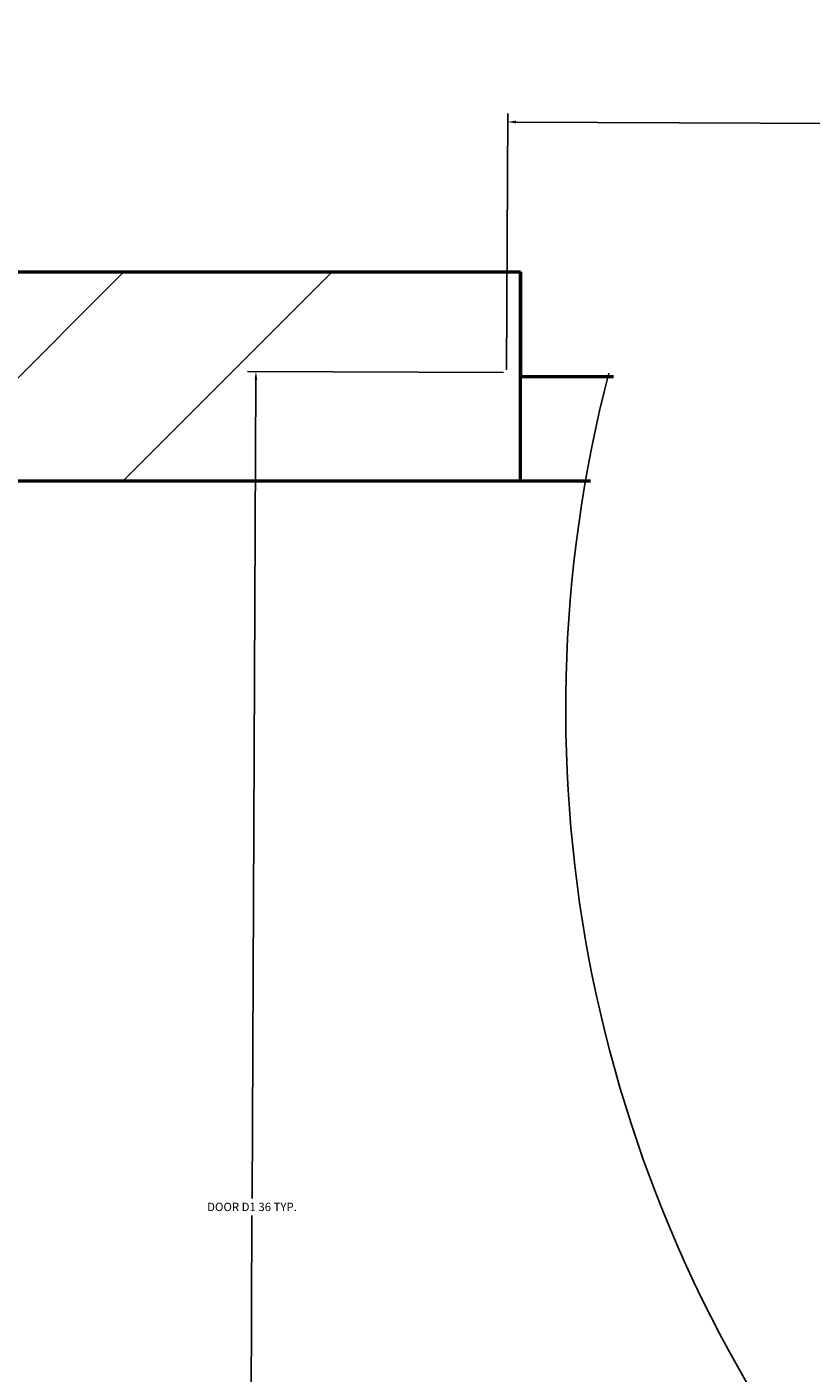
# Model space of a CAD drawing. Units: inches. Extents: x 1901 to 2863, y 888 to 2433.
# Tile 28 of 91: x 2557 to 2573, y 1376 to 1405. Entities that reach past the tile are written whole.
import ezdxf

# ---------------------------------------------------------------- set-up
doc = ezdxf.new("R2010")
doc.units = ezdxf.units.IN
for name, color, linetype, lineweight in [('A-ANNO-DIMS', 2, 'Continuous', 18), ('A-DOOR', 4, 'Continuous', 25), ('A-WALL', 7, 'Continuous', 50), ('A-WALL-PATT', 8, 'Continuous', 13)]:
    doc.layers.add(name, color=color, linetype=linetype, lineweight=lineweight)
doc.styles.get("Standard").update_dxf_attribs({"font": 'arial.ttf'})
doc.dimstyles.get("Standard").update_dxf_attribs({"dimtxt": 0.18, "dimasz": 0.18, "dimexe": 0.18, "dimexo": 0.0625, "dimgap": 0.09, "dimtad": 0, "dimtih": 1, "dimtoh": 1, "dimdec": 4, "dimzin": 0, "dimdsep": 46, "dimtxsty": 'Standard', "dimcen": 0.09, "dimadec": 0, "dimazin": 0, "dimtfac": 1, "dimtdec": 4, "dimtofl": 0, "dimtmove": 0, "dimatfit": 3, "dimfxl": 1, "dimtolj": 1, "dimtzin": 0, "dimarcsym": 0})

# ---------------------------------------------------------------- blocks, each defined once
blk = doc.blocks.new('DOOR-29')
blk.add_arc((-0.004, 7.119), 28.865, 345.6888, 90)
blk = doc.blocks.new('*D31')
at = {"layer": 'A-ANNO-DIMS', "color": 0, "lineweight": -2, "transparency": 16777216}
for p, q in [((2566.77, 1397.965), (2561.253, 1397.99)), ((2561.432, 1397.81), (2561.35, 1380.173)), ((2561.266, 1362.17), (2561.348, 1379.807)), ((2566.603, 1361.965), (2561.085, 1361.991))]:
    blk.add_line(p, q, dxfattribs=at)
at = {"layer": 'A-ANNO-DIMS', "color": 0, "transparency": 16777216}
for points in [[(2561.402, 1397.81), (2561.462, 1397.809), (2561.433, 1397.99)], [(2561.236, 1362.17), (2561.296, 1362.17), (2561.265, 1361.99)]]:
    blk.add_solid(points, dxfattribs=at)
at = {"layer": 'Defpoints', "color": 0, "transparency": 16777216}
for p in [(2566.833, 1397.964), (2561.265, 1361.99), (2566.665, 1361.965)]:
    blk.add_point(p, dxfattribs=at)
at = {"layer": 'A-ANNO-DIMS', "color": 0, "transparency": 16777216, "insert": (2561.349, 1379.99), "char_height": 0.18, "attachment_point": 5}
blk.add_mtext('\\A1;DOOR D1 36 TYP.', dxfattribs=at)
blk = doc.blocks.new('*D32')
at = {"layer": 'A-ANNO-DIMS', "color": 0, "lineweight": -2, "transparency": 16777216}
for p, q in [((2566.833, 1398.027), (2566.858, 1403.544)), ((2567.038, 1403.364), (2581.416, 1403.297)), ((2596.85, 1403.225), (2582.472, 1403.292)), ((2597.005, 1397.887), (2597.03, 1403.404))]:
    blk.add_line(p, q, dxfattribs=at)
at = {"layer": 'A-ANNO-DIMS', "color": 0, "transparency": 16777216}
for points in [[(2567.038, 1403.394), (2567.037, 1403.334), (2566.858, 1403.364)], [(2596.85, 1403.255), (2596.849, 1403.195), (2597.03, 1403.224)]]:
    blk.add_solid(points, dxfattribs=at)
at = {"layer": 'Defpoints', "color": 0, "transparency": 16777216}
for p in [(2566.858, 1403.364), (2566.833, 1397.964), (2597.005, 1397.824)]:
    blk.add_point(p, dxfattribs=at)
at = {"layer": 'A-ANNO-DIMS', "color": 0, "transparency": 16777216, "insert": (2581.944, 1403.294), "char_height": 0.18, "attachment_point": 5}
blk.add_mtext('\\A1;30 TYP.', dxfattribs=at)

msp = doc.modelspace()

# ---------------------------------------------------------------- hatches: boundary and pattern name
at = {"layer": 'A-WALL-PATT'}
h = msp.add_hatch(dxfattribs=at)
h.set_pattern_fill('ANSI32', color=256)
h.paths.add_polyline_path([(2443.926, 2139.888), (2439.426, 2139.888), (2439.426, 2069.348), (2441.676, 2069.348), (2443.926, 2069.348), (2443.926, 2078.634), (2521.926, 2078.634), (2521.926, 2075.067), (2524.176, 2075.067), (2526.426, 2075.067), (2526.426, 2078.634), (2571.755, 2078.634), (2571.755, 2080.884), (2571.755, 2083.134), (2443.926, 2083.134)])
h.paths.add_polyline_path([(2526.426, 2054.634), (2524.176, 2054.634), (2521.926, 2054.634), (2521.926, 2030.634), (2443.926, 2030.634), (2443.926, 2045.348), (2439.426, 2045.348), (2439.426, 1983.867), (2443.926, 1983.867), (2443.926, 2026.134), (2521.926, 2026.134), (2526.426, 2026.134)])
h.paths.add_polyline_path([(2443.926, 1923.867), (2439.426, 1923.867), (2439.426, 1872.634), (2443.926, 1872.634)])
h.paths.add_polyline_path([(2636.233, 1766.134), (2609.926, 1766.134), (2609.926, 1779.785), (2605.426, 1779.785), (2605.426, 1766.134), (2486.614, 1766.134), (2486.614, 1770.671), (2482.114, 1770.671), (2482.114, 1766.134), (2482.114, 1761.634), (2636.233, 1761.634), (2636.233, 1763.884)])
h.paths.add_polyline_path([(2519.536, 1663.384), (2519.536, 1665.634), (2494.926, 1665.634), (2481.831, 1665.634), (2481.831, 1663.384), (2481.831, 1661.134), (2490.426, 1661.134), (2490.426, 1640.157), (2494.926, 1640.157), (2494.926, 1661.134), (2519.536, 1661.134)])
h.paths.add_polyline_path([(2443.926, 1712.134), (2443.926, 1716.634), (2414.464, 1716.634), (2414.464, 1712.134), (2439.426, 1712.134), (2439.426, 1545.507), (2443.926, 1545.507), (2443.926, 1661.134), (2448.475, 1661.134), (2448.475, 1665.634), (2443.926, 1665.634)])
h.paths.add_polyline_path([(2343.426, 1712.134), (2365.525, 1712.134), (2365.525, 1714.384), (2365.525, 1716.634), (2333.871, 1716.634), (2333.871, 1714.384), (2333.871, 1712.134), (2338.926, 1712.134), (2338.926, 1575.634), (2338.926, 1545.507), (2343.426, 1545.507), (2343.426, 1547.507), (2343.426, 1580.134)])
h.paths.add_polyline_path([(2752.926, 1665.634), (2579.536, 1665.634), (2579.536, 1661.134), (2615.926, 1661.134), (2615.926, 1529.134), (2598.931, 1529.134), (2598.931, 1524.634), (2623.127, 1524.634), (2623.127, 1526.884), (2623.127, 1529.134), (2620.426, 1529.134), (2620.426, 1661.134), (2748.426, 1661.134), (2748.426, 1633.499), (2752.926, 1633.499)])
h.paths.add_polyline_path([(2752.926, 1419.929), (2748.426, 1419.929), (2748.426, 1400.134), (2659.426, 1400.134), (2659.426, 1444.333), (2657.176, 1444.333), (2654.926, 1444.333), (2654.926, 1400.134), (2643.649, 1400.134), (2643.649, 1395.634), (2748.426, 1395.634), (2748.426, 1364.035), (2752.926, 1364.035)])
h.paths.add_polyline_path([(2752.926, 1492.878), (2748.426, 1492.878), (2748.426, 1476.634), (2667.426, 1476.634), (2667.426, 1479.71), (2665.176, 1479.71), (2662.926, 1479.71), (2662.926, 1476.634), (2654.926, 1476.634), (2654.926, 1469.536), (2659.426, 1469.536), (2659.426, 1472.134), (2748.426, 1472.134), (2748.426, 1455.929), (2752.926, 1455.929)])
h.paths.add_polyline_path([(2752.926, 1304.035), (2748.426, 1304.035), (2748.426, 1263.634), (2738.66, 1263.634), (2738.66, 1259.134), (2752.926, 1259.134)])
h.paths.add_polyline_path([(2685.926, 1259.134), (2695.49, 1259.134), (2695.49, 1261.384), (2695.49, 1263.634), (2677.837, 1263.634), (2677.837, 1261.384), (2677.837, 1259.134), (2681.426, 1259.134), (2681.426, 1203.634), (2653.277, 1203.634), (2653.277, 1199.134), (2685.926, 1199.134), (2685.926, 1203.634)])
h.paths.add_polyline_path([(2609.426, 1395.634), (2611.848, 1395.634), (2611.848, 1400.134), (2598.888, 1400.134), (2598.888, 1397.884), (2598.888, 1395.634), (2604.926, 1395.634), (2604.926, 1268.134), (2554.726, 1268.134), (2554.726, 1265.884), (2554.726, 1263.634), (2604.926, 1263.634), (2604.926, 1203.634), (2571.306, 1203.634), (2571.306, 1199.134), (2604.926, 1199.134), (2629.277, 1199.134), (2629.277, 1201.384), (2629.277, 1203.634), (2609.426, 1203.634), (2609.426, 1258.634), (2609.426, 1259.134), (2654.804, 1259.134), (2654.804, 1263.634), (2609.426, 1263.634)])
h.paths.add_polyline_path([(2443.926, 1304.035), (2439.426, 1304.035), (2439.426, 1259.134), (2443.926, 1259.134), (2456.16, 1259.134), (2456.16, 1261.384), (2456.16, 1263.634), (2443.926, 1263.634)])
h.paths.add_polyline_path([(2525.426, 1263.634), (2531.778, 1263.634), (2531.778, 1268.134), (2520.926, 1268.134), (2520.926, 1263.634), (2511.409, 1263.634), (2511.409, 1259.134), (2520.926, 1259.134), (2520.926, 1199.134), (2547.306, 1199.134), (2547.306, 1201.384), (2547.306, 1203.634), (2525.426, 1203.634)])
h.paths.add_polyline_path([(2443.926, 1434.842), (2439.426, 1434.842), (2439.426, 1364.035), (2441.676, 1364.035), (2443.926, 1364.035)])
h.paths.add_polyline_path([(2567.134, 1400.134), (2443.926, 1400.134), (2443.926, 1395.634), (2567.134, 1395.634)])
h.paths.add_polyline_path([(2443.926, 1545.507), (2439.426, 1545.507), (2439.426, 1494.842), (2443.926, 1494.842)])
h.paths.add_polyline_path([(2494.926, 1553.349), (2492.676, 1553.349), (2490.426, 1553.349), (2490.426, 1524.634), (2494.926, 1524.634), (2525.936, 1524.634), (2525.936, 1526.884), (2525.936, 1529.134), (2494.926, 1529.134)])
h.paths.add_polyline_path([(2752.926, 1573.499), (2748.426, 1573.499), (2748.426, 1529.134), (2657.759, 1529.134), (2657.759, 1524.634), (2662.926, 1524.634), (2662.926, 1498.631), (2667.426, 1498.631), (2667.426, 1524.634), (2748.426, 1524.634), (2748.426, 1516.878), (2752.926, 1516.878)])
h.paths.add_polyline_path([(2038.602, 2237.418), (2080.174, 2237.418), (2080.174, 2256.075), (2038.602, 2256.075)], flags=9)
h.paths.add_polyline_path([(2292.009, 1062.394), (2539.932, 1062.394), (2539.932, 1099.487), (2292.009, 1099.487)], flags=9)
h.paths.add_polyline_path([(2424.91, 1832.253), (2448.513, 1832.253), (2448.513, 1846.678), (2424.91, 1846.678)], flags=9)
h.paths.add_polyline_path([(2359.076, 1832.253), (2382.678, 1832.253), (2382.678, 1846.678), (2359.076, 1846.678)], flags=9)
h.paths.add_polyline_path([(2352.899, 1684.802), (2367.543, 1684.802), (2367.543, 1697.167), (2352.899, 1697.167)], flags=9)
h.paths.add_polyline_path([(2079.288, 1755.826), (2169.024, 1755.826), (2169.024, 1774.372), (2079.288, 1774.372)], flags=9)
h.paths.add_polyline_path([(2404.09, 1373.857), (2404.09, 1463.593), (2385.544, 1463.593), (2385.544, 1373.857)], flags=9)
h.paths.add_polyline_path([(2268.091, 2236.371), (2309.636, 2236.371), (2309.636, 2255.028), (2268.091, 2255.028)], flags=9)
h.paths.add_polyline_path([(2575.96, 1700.951), (2665.696, 1700.951), (2665.696, 1719.498), (2575.96, 1719.498)], flags=9)
h.paths.add_polyline_path([(2302.962, 1878.474), (2329.524, 1878.474), (2329.524, 1888.777), (2302.962, 1888.777)], flags=9)
h.paths.add_polyline_path([(2097.415, 2240.576), (2126.573, 2240.576), (2126.573, 2259.233), (2097.415, 2259.233)], flags=9)
h.paths.add_polyline_path([(2208.725, 2246.124), (2237.882, 2246.124), (2237.882, 2264.781), (2208.725, 2264.781)], flags=9)
h.paths.add_polyline_path([(2038.147, 1925.958), (2076.987, 1925.958), (2076.987, 1944.615), (2038.147, 1944.615)], flags=9)
h.paths.add_polyline_path([(2239.144, 1926.672), (2288.465, 1926.672), (2288.465, 1945.329), (2239.144, 1945.329)], flags=9)
h.paths.add_polyline_path([(2175.429, 2007.33), (2212.356, 2007.33), (2212.356, 2025.987), (2175.429, 2025.987)], flags=9)
h.paths.add_polyline_path([(2225.034, 2091.794), (2263.875, 2091.794), (2263.875, 2110.451), (2225.034, 2110.451)], flags=9)
h.paths.add_polyline_path([(2035.398, 2098.478), (2074.238, 2098.478), (2074.238, 2117.135), (2035.398, 2117.135)], flags=9)
h.paths.add_polyline_path([(2050.102, 2029.209), (2083.26, 2029.209), (2083.26, 2047.866), (2050.102, 2047.866)], flags=9)
h.paths.add_polyline_path([(2069.677, 1956.719), (2098.835, 1956.719), (2098.835, 1975.376), (2069.677, 1975.376)], flags=9)
h.paths.add_polyline_path([(2328.62, 1753.336), (2361.663, 1753.336), (2361.663, 1771.993), (2328.62, 1771.993)], flags=9)
h.paths.add_polyline_path([(2395.162, 2060.888), (2395.162, 2140.654), (2378.676, 2140.654), (2378.676, 2060.888)], flags=9)
h.paths.add_polyline_path([(2463.728, 2059.02), (2492.886, 2059.02), (2492.886, 2077.677), (2463.728, 2077.677)], flags=9)
h.paths.add_polyline_path([(2458.027, 2181.536), (2496.868, 2181.536), (2496.868, 2200.194), (2458.027, 2200.194)], flags=9)
h.paths.add_polyline_path([(2456.855, 2228.831), (2498.401, 2228.831), (2498.401, 2247.488), (2456.855, 2247.488)], flags=9)
h.paths.add_polyline_path([(2527.577, 2243.074), (2556.735, 2243.074), (2556.735, 2261.731), (2527.577, 2261.731)], flags=9)
h.paths.add_polyline_path([(2694.461, 2232.767), (2736.033, 2232.767), (2736.033, 2251.425), (2694.461, 2251.425)], flags=9)
h.paths.add_polyline_path([(2637.821, 2249.225), (2666.979, 2249.225), (2666.979, 2267.882), (2637.821, 2267.882)], flags=9)
h.paths.add_polyline_path([(2623.687, 2183.541), (2662.528, 2183.541), (2662.528, 2202.199), (2623.687, 2202.199)], flags=9)
h.paths.add_polyline_path([(2691.965, 2021.5), (2725.124, 2021.5), (2725.124, 2040.157), (2691.965, 2040.157)], flags=9)
h.paths.add_polyline_path([(2621.043, 1975.912), (2662.335, 1975.912), (2662.335, 1994.569), (2621.043, 1994.569)], flags=9)
h.paths.add_polyline_path([(2479.032, 1927.62), (2519.844, 1927.62), (2519.844, 1946.277), (2479.032, 1946.277)], flags=9)
h.paths.add_polyline_path([(2670.941, 1849.076), (2716.005, 1849.076), (2716.005, 1867.734), (2670.941, 1867.734)], flags=9)
h.paths.add_polyline_path([(2523.613, 1782.956), (2550.175, 1782.956), (2550.175, 1793.26), (2523.613, 1793.26)], flags=9)
h.paths.add_polyline_path([(2450.841, 1207.331), (2492.386, 1207.331), (2492.386, 1225.989), (2450.841, 1225.989)], flags=9)
h.paths.add_polyline_path([(2527.751, 1203.841), (2556.908, 1203.841), (2556.908, 1222.499), (2527.751, 1222.499)], flags=9)
h.paths.add_polyline_path([(2639.111, 1207.2), (2668.268, 1207.2), (2668.268, 1225.857), (2639.111, 1225.857)], flags=9)
h.paths.add_polyline_path([(2692.594, 1218.965), (2734.167, 1218.965), (2734.167, 1237.623), (2692.594, 1237.623)], flags=9)
h.paths.add_polyline_path([(2669.266, 1366.329), (2708.106, 1366.329), (2708.106, 1384.987), (2669.266, 1384.987)], flags=25)
h.paths.add_polyline_path([(2463.313, 1358.031), (2502.153, 1358.031), (2502.153, 1376.688), (2463.313, 1376.688)], flags=9)
h.paths.add_polyline_path([(2494.725, 1449.963), (2531.652, 1449.963), (2531.652, 1468.62), (2494.725, 1468.62)], flags=9)
h.paths.add_polyline_path([(2675.565, 1422.157), (2708.724, 1422.157), (2708.724, 1440.815), (2675.565, 1440.815)], flags=25)
h.paths.add_polyline_path([(2685.634, 1493.891), (2714.792, 1493.891), (2714.792, 1512.548), (2685.634, 1512.548)], flags=9)
h.paths.add_polyline_path([(2686.805, 1529.913), (2725.645, 1529.913), (2725.645, 1548.57), (2686.805, 1548.57)], flags=25)
h.paths.add_polyline_path([(2503.651, 1537.991), (2552.972, 1537.991), (2552.972, 1556.648), (2503.651, 1556.648)], flags=9)
h.paths.add_polyline_path([(2291.713, 1643.504), (2318.275, 1643.504), (2318.275, 1653.807), (2291.713, 1653.807)], flags=9)
h.paths.add_polyline_path([(2450.626, 1610.52), (2477.189, 1610.52), (2477.189, 1620.824), (2450.626, 1620.824)], flags=9)
h.paths.add_polyline_path([(2359.985, 1551.814), (2422.253, 1551.814), (2422.253, 1562.117), (2359.985, 1562.117)], flags=9)
h.paths.add_polyline_path([(2280.106, 1249.006), (2321.651, 1249.006), (2321.651, 1267.663), (2280.106, 1267.663)], flags=9)
h.paths.add_polyline_path([(2164.057, 1274.232), (2193.215, 1274.232), (2193.215, 1292.889), (2164.057, 1292.889)], flags=9)
h.paths.add_polyline_path([(2118.21, 1277.694), (2151.252, 1277.694), (2151.252, 1296.351), (2118.21, 1296.351)], flags=9)
h.paths.add_polyline_path([(2031.946, 1268.529), (2073.519, 1268.529), (2073.519, 1287.187), (2031.946, 1287.187)], flags=9)
h.paths.add_polyline_path([(2050.199, 1409.079), (2089.04, 1409.079), (2089.04, 1427.736), (2050.199, 1427.736)], flags=9)
h.paths.add_polyline_path([(2243.743, 1421.032), (2282.584, 1421.032), (2282.584, 1439.689), (2243.743, 1439.689)], flags=9)
h.paths.add_polyline_path([(2190.746, 1509.769), (2231.558, 1509.769), (2231.558, 1528.426), (2190.746, 1528.426)], flags=9)
h.paths.add_polyline_path([(2058.392, 1475.415), (2091.55, 1475.415), (2091.55, 1494.073), (2058.392, 1494.073)], flags=9)
h.paths.add_polyline_path([(2062.447, 1553.09), (2091.605, 1553.09), (2091.605, 1571.747), (2062.447, 1571.747)], flags=9)
h.paths.add_polyline_path([(2219.524, 1590.365), (2266.147, 1590.365), (2266.147, 1609.022), (2219.524, 1609.022)], flags=9)
h.paths.add_polyline_path([(2041.072, 1584.188), (2079.912, 1584.188), (2079.912, 1602.845), (2041.072, 1602.845)], flags=9)

# ---------------------------------------------------------------- linework, layer by layer
at = {"layer": 'A-WALL'}
for p, q in [((2443.926, 1400.134), (2567.134, 1400.134)), ((2567.134, 1395.634), (2567.134, 1400.134)), ((2567.134, 1400.134), (2567.134, 1397.884)), ((2567.134, 1397.884), (2569.134, 1397.884)), ((2443.926, 1395.634), (2568.638, 1395.634))]:
    msp.add_line(p, q, dxfattribs=at)

# ---------------------------------------------------------------- block references
at = {"layer": 'A-DOOR', "rotation": 179.7338121645225}
msp.add_blockref('DOOR-29', (2597.001, 1397.808), dxfattribs=at)

# ---------------------------------------------------------------- dimensions: what is measured, and where the dimension line sits
at = {"layer": 'A-ANNO-DIMS'}
for base, p1, p2, angle, text, picture, middle in [((2566.858, 1403.364), (2597.005, 1397.824), (2566.833, 1397.964), 179.7338, '<> TYP.', '*D32', (2581.944, 1403.294)), ((2561.265, 1361.99), (2566.833, 1397.964), (2566.665, 1361.965), 269.7338, 'DOOR D1 <> TYP.', '*D31', (2561.349, 1379.99))]:
    dim = msp.add_linear_dim(base=base, p1=p1, p2=p2, angle=angle, text=text, dimstyle='Standard', override={"dimdec": 0, "dimlfac": 1, "dimrnd": 0, "dimzin": 0, "dimdsep": 46, "dimlunit": 2}, dxfattribs=at)
    dim.commit()
    dim.dimension.update_dxf_attribs({"geometry": picture, "text_midpoint": middle})

doc.saveas('drawing.dxf')
